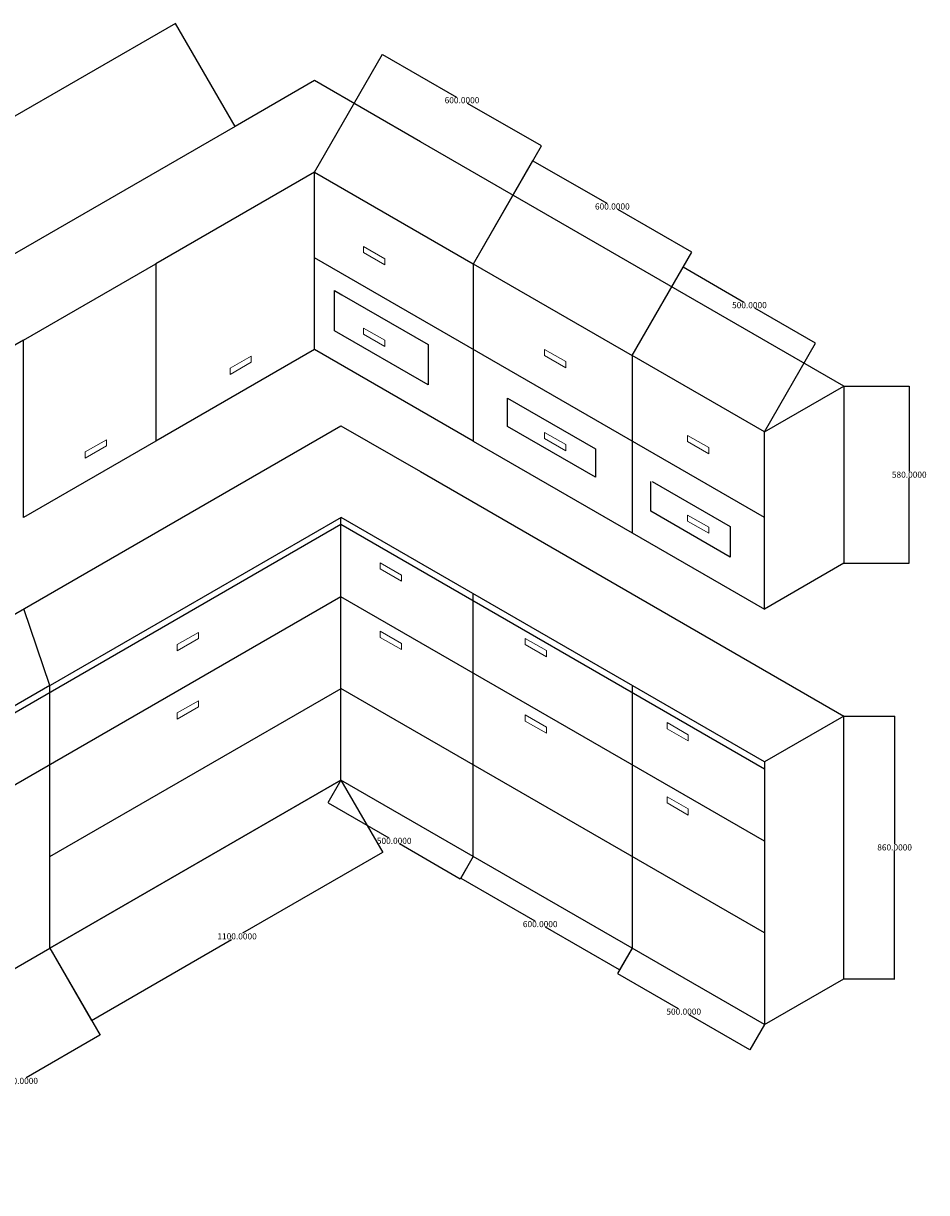
# Model space of a CAD drawing. Units: millimetres. Extents: x -886 to 3895, y -26 to 3802.
# Tile 2 of 2: x 939 to 3895, y -26 to 3802. Entities that reach past the tile are written whole.
import ezdxf

# ---------------------------------------------------------------- set-up
doc = ezdxf.new("R2010")
doc.units = ezdxf.units.MM
doc.header["$MEASUREMENT"] = 0
for name, color, linetype, lineweight in [('A-ANNO-DIMS', 2, 'Continuous', 18), ('A-FURN', 7, 'Continuous', 25), ('A-FURN-HDWR', 8, 'Continuous', 18)]:
    doc.layers.add(name, color=color, linetype=linetype, lineweight=lineweight)
doc.styles.get("Standard").update_dxf_attribs({"font": 'arial.ttf'})
doc.dimstyles.get("Standard").update_dxf_attribs({"dimtxt": 0.18, "dimasz": 0.18, "dimexe": 0.18, "dimexo": 0.0625, "dimgap": 0.09, "dimtad": 0, "dimtih": 1, "dimtoh": 1, "dimdec": 4, "dimzin": 0, "dimdsep": 46, "dimtxsty": 'Standard', "dimcen": 0.09, "dimadec": 0, "dimazin": 0, "dimtfac": 1, "dimtdec": 4, "dimtofl": 0, "dimtmove": 0, "dimatfit": 3, "dimfxl": 1, "dimtolj": 1, "dimtzin": 0, "dimarcsym": 0})

# ---------------------------------------------------------------- blocks, each defined once
blk = doc.blocks.new('*D2')
at = {"layer": 'A-ANNO-DIMS', "color": 0, "lineweight": -2, "transparency": 16777216}
for p, q in [((3624.1, 1534.3), (3790.4, 1534.3)), ((3790.2, 1534.1), (3790.2, 1114.6)), ((3790.2, 674.5), (3790.2, 1094)), ((3624.1, 674.3), (3790.4, 674.3))]:
    blk.add_line(p, q, dxfattribs=at)
at = {"layer": 'A-ANNO-DIMS', "color": 0, "transparency": 16777216}
for points in [[(3790.1, 1534.1), (3790.2, 1534.1), (3790.2, 1534.3)], [(3790.1, 674.5), (3790.2, 674.5), (3790.2, 674.3)]]:
    blk.add_solid(points, dxfattribs=at)
at = {"layer": 'Defpoints', "color": 0, "transparency": 16777216}
for p in [(3624.1, 1534.3), (3624.1, 674.3), (3790.2, 674.3)]:
    blk.add_point(p, dxfattribs=at)
at = {"layer": 'A-ANNO-DIMS', "color": 0, "transparency": 16777216, "insert": (3790.2, 1104.3), "char_height": 20, "attachment_point": 5}
blk.add_mtext('\\A1;860.0000', dxfattribs=at)
blk = doc.blocks.new('*D3')
at = {"layer": 'A-ANNO-DIMS', "color": 0, "lineweight": -2, "transparency": 16777216}
for p, q in [((3624.1, 2614.3), (3838.2, 2614.3)), ((3838.1, 2614.1), (3838.1, 2334.6)), ((3838.1, 2034.5), (3838.1, 2314)), ((3624.1, 2034.3), (3838.2, 2034.3))]:
    blk.add_line(p, q, dxfattribs=at)
at = {"layer": 'A-ANNO-DIMS', "color": 0, "transparency": 16777216}
for points in [[(3838, 2614.1), (3838.1, 2614.1), (3838.1, 2614.3)], [(3838, 2034.5), (3838.1, 2034.5), (3838.1, 2034.3)]]:
    blk.add_solid(points, dxfattribs=at)
at = {"layer": 'Defpoints', "color": 0, "transparency": 16777216}
for p in [(3624.1, 2614.3), (3624.1, 2034.3), (3838.1, 2034.3)]:
    blk.add_point(p, dxfattribs=at)
at = {"layer": 'A-ANNO-DIMS', "color": 0, "transparency": 16777216, "insert": (3838.1, 2324.3), "char_height": 20, "attachment_point": 5}
blk.add_mtext('\\A1;580.0000', dxfattribs=at)
blk = doc.blocks.new('*D4')
at = {"layer": 'A-ANNO-DIMS', "color": 0, "lineweight": -2, "transparency": 16777216}
for p, q in [((2931.3, 2714.3), (3098.7, 3004.4)), ((3098.8, 3004.1), (3297.3, 2889.5)), ((3531.5, 2754.3), (3333, 2868.9)), ((3364.3, 2464.3), (3531.7, 2754.4))]:
    blk.add_line(p, q, dxfattribs=at)
at = {"layer": 'A-ANNO-DIMS', "color": 0, "transparency": 16777216}
for points in [[(3098.8, 3004.1), (3098.8, 3004.1), (3098.6, 3004.2)], [(3531.5, 2754.3), (3531.5, 2754.3), (3531.6, 2754.2)]]:
    blk.add_solid(points, dxfattribs=at)
at = {"layer": 'Defpoints', "color": 0, "transparency": 16777216}
for p in [(3531.6, 2754.2), (2931.2, 2714.3), (3364.3, 2464.3)]:
    blk.add_point(p, dxfattribs=at)
at = {"layer": 'A-ANNO-DIMS', "color": 0, "transparency": 16777216, "insert": (3315.1, 2879.2), "char_height": 20, "attachment_point": 5}
blk.add_mtext('\\A1;500.0000', dxfattribs=at)
blk = doc.blocks.new('*D5')
at = {"layer": 'A-ANNO-DIMS', "color": 0, "lineweight": -2, "transparency": 16777216}
for p, q in [((2411.7, 3014.3), (2606.8, 3352.3)), ((2606.9, 3352.1), (2848.7, 3212.5)), ((3126.2, 3052.3), (2884.4, 3191.9)), ((2931.3, 2714.3), (3126.4, 3052.3))]:
    blk.add_line(p, q, dxfattribs=at)
at = {"layer": 'A-ANNO-DIMS', "color": 0, "transparency": 16777216}
for points in [[(2606.9, 3352.1), (2606.9, 3352.1), (2606.7, 3352.2)], [(3126.2, 3052.3), (3126.2, 3052.3), (3126.3, 3052.2)]]:
    blk.add_solid(points, dxfattribs=at)
at = {"layer": 'Defpoints', "color": 0, "transparency": 16777216}
for p in [(3126.3, 3052.2), (2411.6, 3014.3), (2931.2, 2714.3)]:
    blk.add_point(p, dxfattribs=at)
at = {"layer": 'A-ANNO-DIMS', "color": 0, "transparency": 16777216, "insert": (2866.5, 3202.2), "char_height": 20, "attachment_point": 5}
blk.add_mtext('\\A1;600.0000', dxfattribs=at)
blk = doc.blocks.new('*D6')
at = {"layer": 'A-ANNO-DIMS', "color": 0, "lineweight": -2, "transparency": 16777216}
for p, q in [((1892, 3314.3), (2114.9, 3700.3)), ((2114.9, 3700), (2356.8, 3560.4)), ((2634.3, 3400.2), (2392.4, 3539.8)), ((2411.7, 3014.3), (2634.5, 3400.3))]:
    blk.add_line(p, q, dxfattribs=at)
at = {"layer": 'A-ANNO-DIMS', "color": 0, "transparency": 16777216}
for points in [[(2115, 3700.1), (2114.9, 3700), (2114.8, 3700.1)], [(2634.3, 3400.3), (2634.2, 3400.2), (2634.4, 3400.1)]]:
    blk.add_solid(points, dxfattribs=at)
at = {"layer": 'Defpoints', "color": 0, "transparency": 16777216}
for p in [(2634.4, 3400.1), (1892, 3314.3), (2411.6, 3014.3)]:
    blk.add_point(p, dxfattribs=at)
at = {"layer": 'A-ANNO-DIMS', "color": 0, "transparency": 16777216, "insert": (2374.6, 3550.1), "char_height": 20, "attachment_point": 5}
blk.add_mtext('\\A1;600.0000', dxfattribs=at)
blk = doc.blocks.new('*D7')
at = {"layer": 'A-ANNO-DIMS', "color": 0, "lineweight": -2, "transparency": 16777216}
for p, q in [((1437.4, 3801.3), (546.1, 3286.7)), ((1632.2, 3464.3), (1437.5, 3801.5)), ((-380.9, 2751.4), (510.4, 3266.1)), ((-186.5, 2414.3), (-381.2, 2751.5))]:
    blk.add_line(p, q, dxfattribs=at)
at = {"layer": 'A-ANNO-DIMS', "color": 0, "transparency": 16777216}
for points in [[(1437.4, 3801.3), (1437.5, 3801.2), (1437.6, 3801.4)], [(-380.9, 2751.5), (-380.9, 2751.4), (-381.1, 2751.4)]]:
    blk.add_solid(points, dxfattribs=at)
at = {"layer": 'Defpoints', "color": 0, "transparency": 16777216}
for p in [(1632.2, 3464.3), (-381.1, 2751.4), (-186.4, 2414.3)]:
    blk.add_point(p, dxfattribs=at)
at = {"layer": 'A-ANNO-DIMS', "color": 0, "transparency": 16777216, "insert": (528.3, 3276.4), "char_height": 20, "attachment_point": 5}
blk.add_mtext('\\A1;2100.0000', dxfattribs=at)
blk = doc.blocks.new('*D9')
at = {"layer": 'A-ANNO-DIMS', "color": 0, "lineweight": -2, "transparency": 16777216}
for p, q in [((1026, 774.2), (1190.2, 489.9)), ((506.4, 474.2), (670.6, 189.9)), ((1189.9, 489.9), (948.1, 350.3)), ((670.6, 190.1), (912.4, 329.7))]:
    blk.add_line(p, q, dxfattribs=at)
at = {"layer": 'A-ANNO-DIMS', "color": 0, "transparency": 16777216}
for points in [[(1189.9, 490), (1190, 489.9), (1190.1, 490)], [(670.6, 190.1), (670.7, 190.1), (670.5, 190)]]:
    blk.add_solid(points, dxfattribs=at)
at = {"layer": 'Defpoints', "color": 0, "transparency": 16777216}
for p in [(1026, 774.3), (506.4, 474.3), (1190.1, 490)]:
    blk.add_point(p, dxfattribs=at)
at = {"layer": 'A-ANNO-DIMS', "color": 0, "transparency": 16777216, "insert": (930.3, 340), "char_height": 20, "attachment_point": 5}
blk.add_mtext('\\A1;600.0000', dxfattribs=at)
blk = doc.blocks.new('*D10')
at = {"layer": 'A-ANNO-DIMS', "color": 0, "lineweight": -2, "transparency": 16777216}
for p, q in [((1978.6, 1324.2), (2115.1, 1088)), ((2114.8, 1088), (1656.5, 823.4)), ((1026, 774.2), (1162.4, 538)), ((1162.5, 538.2), (1620.8, 802.8))]:
    blk.add_line(p, q, dxfattribs=at)
at = {"layer": 'A-ANNO-DIMS', "color": 0, "transparency": 16777216}
for points in [[(2114.8, 1088.1), (2114.8, 1088), (2115, 1088.1)], [(1162.5, 538.2), (1162.5, 538.2), (1162.3, 538.1)]]:
    blk.add_solid(points, dxfattribs=at)
at = {"layer": 'Defpoints', "color": 0, "transparency": 16777216}
for p in [(1978.6, 1324.3), (2115, 1088.1), (1026, 774.3)]:
    blk.add_point(p, dxfattribs=at)
at = {"layer": 'A-ANNO-DIMS', "color": 0, "transparency": 16777216, "insert": (1638.6, 813.1), "char_height": 20, "attachment_point": 5}
blk.add_mtext('\\A1;1100.0000', dxfattribs=at)
blk = doc.blocks.new('*D11')
at = {"layer": 'A-ANNO-DIMS', "color": 0, "lineweight": -2, "transparency": 16777216}
for p, q in [((1978.6, 1324.2), (1936.1, 1250.6)), ((1936.3, 1250.6), (2134.8, 1136)), ((2369, 1000.8), (2170.5, 1115.4)), ((2411.6, 1074.2), (2369.1, 1000.6))]:
    blk.add_line(p, q, dxfattribs=at)
at = {"layer": 'A-ANNO-DIMS', "color": 0, "transparency": 16777216}
for points in [[(1936.3, 1250.6), (1936.3, 1250.6), (1936.1, 1250.7)], [(2369, 1000.8), (2369, 1000.8), (2369.2, 1000.7)]]:
    blk.add_solid(points, dxfattribs=at)
at = {"layer": 'Defpoints', "color": 0, "transparency": 16777216}
for p in [(1978.6, 1324.3), (1936.1, 1250.7), (2411.6, 1074.3)]:
    blk.add_point(p, dxfattribs=at)
at = {"layer": 'A-ANNO-DIMS', "color": 0, "transparency": 16777216, "insert": (2152.7, 1125.7), "char_height": 20, "attachment_point": 5}
blk.add_mtext('\\A1;500.0000', dxfattribs=at)
blk = doc.blocks.new('*D12')
at = {"layer": 'A-ANNO-DIMS', "color": 0, "lineweight": -2, "transparency": 16777216}
for p, q in [((2411.6, 1074.2), (2370.6, 1003.1)), ((2370.8, 1003.2), (2612.6, 863.6)), ((2890.1, 703.4), (2648.3, 843)), ((2931.2, 774.2), (2890.2, 703.1))]:
    blk.add_line(p, q, dxfattribs=at)
at = {"layer": 'A-ANNO-DIMS', "color": 0, "transparency": 16777216}
for points in [[(2370.8, 1003.2), (2370.8, 1003.2), (2370.6, 1003.3)], [(2890.1, 703.4), (2890.1, 703.4), (2890.3, 703.3)]]:
    blk.add_solid(points, dxfattribs=at)
at = {"layer": 'Defpoints', "color": 0, "transparency": 16777216}
for p in [(2411.6, 1074.3), (2370.6, 1003.3), (2931.2, 774.3)]:
    blk.add_point(p, dxfattribs=at)
at = {"layer": 'A-ANNO-DIMS', "color": 0, "transparency": 16777216, "insert": (2630.5, 853.3), "char_height": 20, "attachment_point": 5}
blk.add_mtext('\\A1;600.0000', dxfattribs=at)
blk = doc.blocks.new('*D13')
at = {"layer": 'A-ANNO-DIMS', "color": 0, "lineweight": -2, "transparency": 16777216}
for p, q in [((2931.2, 774.2), (2883.5, 691.5)), ((2883.7, 691.6), (3082.2, 577)), ((3316.4, 441.8), (3117.9, 556.4)), ((3364.2, 524.2), (3316.5, 441.5))]:
    blk.add_line(p, q, dxfattribs=at)
at = {"layer": 'A-ANNO-DIMS', "color": 0, "transparency": 16777216}
for points in [[(2883.7, 691.6), (2883.7, 691.6), (2883.6, 691.7)], [(3316.4, 441.8), (3316.4, 441.7), (3316.6, 441.7)]]:
    blk.add_solid(points, dxfattribs=at)
at = {"layer": 'Defpoints', "color": 0, "transparency": 16777216}
for p in [(2931.2, 774.3), (2883.6, 691.7), (3364.3, 524.3)]:
    blk.add_point(p, dxfattribs=at)
at = {"layer": 'A-ANNO-DIMS', "color": 0, "transparency": 16777216, "insert": (3100.1, 566.7), "char_height": 20, "attachment_point": 5}
blk.add_mtext('\\A1;500.0000', dxfattribs=at)
blk = doc.blocks.new('CAB-HANDLE-A')
blk.add_lwpolyline([(69.3, 0), (69.3, 20), (0, 60), (0, 40)], close=True)
blk = doc.blocks.new('CAB-HANDLE-B')
blk.add_lwpolyline([(69.3, 40), (69.3, 60), (0, 20), (0, 0)], close=True)

msp = doc.modelspace()

# ---------------------------------------------------------------- linework, layer by layer
at = {"layer": 'A-FURN'}
for p, q in [((1025.99022, 1074.27277), (1979.11124, 1624.55745)), ((3364.25884, 824.27279), (1978.6182, 1624.27279))]:
    msp.add_line(p, q, dxfattribs=at)
for points in [[(3624.06646, 2614.27279), (2238.42582, 3414.27279), (1892.01566, 3614.27279), (1632.20803, 3464.27279), (-186.44531, 2414.27279)], [(1892.01566, 2734.27279), (1892.01566, 3314.27279), (1372.40041, 3014.27279)], [(1892.01566, 3314.27279), (2411.6309, 3014.27279), (2931.24614, 2714.27279)], [(2411.6309, 3014.27279), (2411.6309, 2434.27279), (2931.24614, 2134.27279), (3364.25884, 1884.27279), (3364.25884, 2184.27279), (1892.01566, 3034.27279)], [(939.38771, 2764.27279), (1372.40041, 3014.27279), (1372.40041, 2434.27279)], [(2411.6309, 2434.27279), (1892.01566, 2734.27279), (1372.40041, 2434.27279), (939.38771, 2184.27279), (939.38771, 2764.27279), (419.77247, 2464.27279), (73.36231, 2264.27279), (-186.44531, 2414.27279), (-186.44531, 1994.27279)], [(3364.25884, 2464.27279), (3624.06646, 2614.27279), (3624.06646, 2034.27279), (3364.25884, 1884.27279), (3364.25884, 2464.27279), (2931.24614, 2714.27279), (2931.24614, 2134.27279)], [(159.96485, 1134.27286), (159.96485, 1434.27286), (1978.6182, 2484.27286), (2238.42582, 2334.27286), (3624.06646, 1534.27286)], [(2996.61217, 2302.11018), (3252.44999, 2154.40215), (3252.44999, 2054.50072), (2992.25561, 2204.72401), (2992.25561, 2302.11018)], [(3364.25884, 1384.27279), (1979.32525, 2183.86457), (1027.40226, 1634.27158)], [(3364.25884, 524.27279), (2931.24614, 774.27279), (2411.6309, 1074.27279), (1978.6182, 1324.27279), (1978.6182, 2183.45636)], [(159.96485, 1111.93531), (1978.6182, 2161.93531), (3364.25884, 1361.93531)], [(1025.99022, 1634.27284), (506.37498, 1334.27284), (506.37498, 474.27284), (159.96485, 274.27279), (159.96485, 1894.27279), (-99.84277, 2044.27279), (-619.45802, 1744.27279), (-619.45802, 124.27279), (-359.65039, -25.72721), (-359.65039, 1594.27279)], [(3364.25884, 1124.27279), (1978.6182, 1924.27279), (159.96485, 874.27279)], [(2931.24614, 1634.27279), (2931.24614, 774.27279), (2411.6309, 1074.27279), (2411.6309, 1934.27279)], [(1978.61823, 1324.27274), (1025.99022, 774.27284), (1025.99022, 1634.27284), (940.93853, 1885.16822)], [(-359.65039, -25.72721), (159.96485, 274.27279), (506.37501, 474.27279), (1025.99025, 774.27279), (1978.6182, 1324.27279)]]:
    msp.add_lwpolyline(points, dxfattribs=at)
for points in [[(2263.99694, 2749.9201), (2263.99694, 2618.38817), (1957.81919, 2795.15997), (1957.81919, 2926.6919), (1981.00237, 2913.30709)], [(2810.9584, 2409.29744), (2810.9584, 2316.04163), (2523.57896, 2481.96022), (2523.57896, 2575.21604)], [(3364.25884, 524.27279), (3624.06646, 674.27279), (3624.06646, 1534.27279), (3364.25884, 1384.27279)]]:
    msp.add_lwpolyline(points, close=True, dxfattribs=at)

# ---------------------------------------------------------------- block references
at = {"layer": 'A-FURN-HDWR'}
for name, p in [('CAB-HANDLE-A', (2052.68855, 3011.2814)), ('CAB-HANDLE-A', (2052.68855, 2744.35833)), ('CAB-HANDLE-A', (2644.648, 2674.333)), ('CAB-HANDLE-A', (2644.648, 2402.59038)), ('CAB-HANDLE-A', (3112.7973, 2393.02938)), ('CAB-HANDLE-A', (3112.7973, 2132.30426)), ('CAB-HANDLE-A', (2107.21759, 1975.90681)), ('CAB-HANDLE-B', (1442.705, 1747.962)), ('CAB-HANDLE-A', (2107.21759, 1751.69773)), ('CAB-HANDLE-A', (2581.72553, 1728.52871)), ('CAB-HANDLE-B', (1442.705, 1524.49939)), ('CAB-HANDLE-A', (2581.72553, 1477.74044)), ('CAB-HANDLE-A', (3045.50705, 1452.58948)), ('CAB-HANDLE-A', (3045.50705, 1209.97605))]:
    msp.add_blockref(name, p, dxfattribs=at)
at = {"layer": 'A-FURN-HDWR', "extrusion": (0, 0, -1), "zscale": -1, "rotation": 180}
for p in [(-1615.8107, 2712.47763), (-1141.71452, 2438.75807)]:
    msp.add_blockref('CAB-HANDLE-A', p, dxfattribs=at)

# ---------------------------------------------------------------- dimensions: what is measured, and where the dimension line sits
at = {"layer": 'A-ANNO-DIMS'}
for p1, p2, distance, picture, middle in [((1632.20803, 3464.27279), (-186.44531, 2414.27279), -389.2306, '*D7', (528.26606, 3276.35638)), ((1892.01566, 3314.27279), (2411.6309, 3014.27279), 445.55657, '*D6', (2374.60156, 3550.1361)), ((2411.6309, 3014.27279), (2931.24614, 2714.27279), 390.18881, '*D5', (2866.53293, 3202.18621)), ((2931.24614, 2714.27279), (3364.25884, 2464.27279), 334.77992, '*D4', (3315.14245, 2879.2007)), ((1025.99022, 774.27284), (1978.6182, 1324.27279), -272.68831, '*D10', (1638.64835, 813.1178)), ((2411.6309, 1074.27279), (1978.6182, 1324.27279), 84.93867, '*D11', (2152.65521, 1125.71374)), ((2931.24614, 774.27279), (2411.6309, 1074.27279), 81.96354, '*D12', (2630.45675, 853.29028)), ((506.37498, 474.27284), (1025.99025, 774.27279), -328.21158, '*D9', (930.28837, 340.03324)), ((3364.25884, 524.27279), (2931.24614, 774.27279), 95.36338, '*D13', (3100.0708, 566.68568))]:
    dim = msp.add_aligned_dim(p1=p1, p2=p2, distance=distance, dimstyle='Standard', override={"dimtxt": 20, "dimclrd": 0, "dimclre": 0, "dimclrt": 0}, dxfattribs=at)
    dim.commit()
    dim.dimension.update_dxf_attribs({"geometry": picture, "text_midpoint": middle})
for base, p1, p2, picture, middle in [((3838.058, 2034.27279), (3624.06646, 2614.27279), (3624.06646, 2034.27279), '*D3', (3838.058, 2324.27279)), ((3790.17923, 674.27279), (3624.06646, 1534.27279), (3624.06646, 674.27279), '*D2', (3790.17923, 1104.27279))]:
    dim = msp.add_linear_dim(base=base, p1=p1, p2=p2, angle=90, dimstyle='Standard', override={"dimtxt": 20, "dimclrd": 0, "dimclre": 0, "dimclrt": 0}, dxfattribs=at)
    dim.commit()
    dim.dimension.update_dxf_attribs({"geometry": picture, "text_midpoint": middle})

doc.saveas('drawing.dxf')
